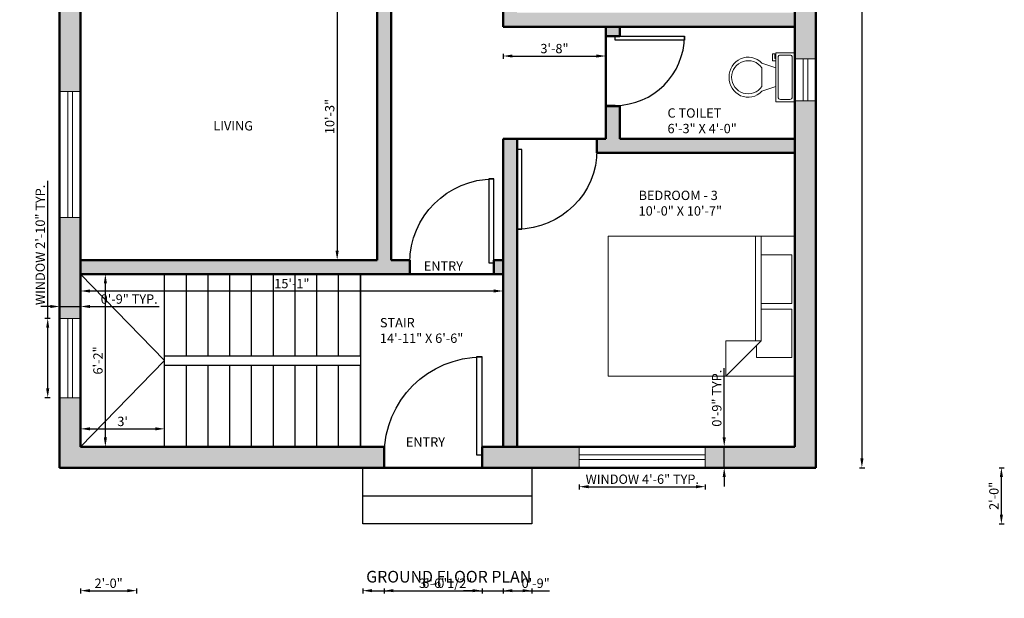
# Model space of a CAD drawing. Units: inches. Extents: x -33 to 405, y -509 to 99.
# Tile 1 of 2: x -16 to 405, y -509 to -262. Entities that reach past the tile are written whole.
import ezdxf

# ---------------------------------------------------------------- set-up
doc = ezdxf.new("R2010")
doc.units = ezdxf.units.IN
for name, color, linetype, lineweight in [('A-ANNO-DIMS', 2, 'Continuous', 18), ('A-ANNO-TEXT', 7, 'Continuous', 25), ('A-AREA-IDEN', 7, 'Continuous', 18), ('A-DOOR', 4, 'Continuous', 25), ('A-FLOR-FIXT', 8, 'Continuous', 18), ('A-FLOR-STRS', 7, 'Continuous', 25), ('A-FURN', 9, 'Continuous', 18), ('A-GLAZ', 6, 'Continuous', 18), ('A-WALL', 7, 'Continuous', 50), ('A-WALL-PATT', 251, 'Continuous', 13)]:
    doc.layers.add(name, color=color, linetype=linetype, lineweight=lineweight)
doc.styles.get("Standard").update_dxf_attribs({"font": 'arial.ttf'})
doc.dimstyles.new('ISO-25', dxfattribs={"dimtxt": 4, "dimasz": 4, "dimexe": 1.25, "dimexo": 0.625, "dimtad": 1, "dimlunit": 3, "dimtxsty": 'Standard', "dimcen": 2.5, "dimadec": 0, "dimazin": 0, "dimtfac": 1, "dimtmove": 0, "dimatfit": 3, "dimfxl": 1, "dimfxlon": 1, "dimarcsym": 0})

# ---------------------------------------------------------------- blocks, each defined once
blk = doc.blocks.new('*U2')
for p, q in [((9.5, -6), (9.5, -2)), ((-8, -8.5), (-8, -8)), ((-7, -8), (-7, -9.5)), ((-4, -8), (-6, -14)), ((4, -8), (6, -14)), ((-10, -8.5), (-8, -8.5)), ((-10, -9.5), (-10, -8.5)), ((-7, -9.5), (-10, -9.5)), ((4, -14), (-4, -14))]:
    blk.add_line(p, q)
blk.add_lwpolyline([(10.5, -8), (10.5, 0), (-10.5, 0), (-10.5, -8)], close=True)
for points in [[(-9.5, -2), (-9.5, -6)], [(8.5, -1), (-8.5, -1)], [(-8.5, -7), (8.5, -7)]]:
    blk.add_lwpolyline(points)
for centre, radius, start, end in [((-8.625, -1.875), 0.8839, 81.8699, 188.1301), ((8.625, -1.875), 0.8839, 351.8699, 98.1301), ((-8.625, -6.125), 0.8839, 171.869898, 278.1301), ((8.625, -6.125), 0.8839, 261.8699, 8.1301), ((-0.4772, -19.9188), 8.0953, 133.01722, 273.38), ((0.0374, -19.8731), 7.127, 124.50543, 269.7), ((-0.0373, -19.8731), 7.127, 270.3, 55.4946), ((0.4773, -19.9188), 8.0953, 266.62, 46.9828)]:
    blk.add_arc(centre, radius, start, end)
blk = doc.blocks.new('*U4')
for p, q in [((0, 0), (0, -100)), ((750, 0), (750, -100))]:
    blk.add_line(p, q)
blk.add_lwpolyline([(0, 0), (0, 750), (43.75, 750), (43.75, 0)], close=True)
blk.add_arc((0, 0), 750, 0, 90)
blk = doc.blocks.new('Bed - Queen')
for p, q in [((0, -80.00003), (0, 0)), ((0, 0), (59.99999, 0)), ((59.99999, 0), (59.99999, -80.00003)), ((7.99999, -1.2), (28.79998, -1.2)), ((7.99999, -14.4), (7.99999, -1.2)), ((28.79998, -1.2), (28.79998, -14.4)), ((31.19999, -1.2), (51.99999, -1.2)), ((31.19999, -14.4), (31.19999, -1.2)), ((51.99999, -1.2), (51.99999, -16.4)), ((0, -14.4), (44.8, -14.4)), ((44.8, -16.8), (0, -16.8)), ((59.99999, -29.6), (44.8, -14.4)), ((44.8, -14.4), (44.8, -29.6)), ((51.99999, -16.4), (46.79936, -16.4)), ((44.8, -29.6), (59.99999, -29.6)), ((59.99999, -80.00003), (0, -80.00003))]:
    blk.add_line(p, q)
blk = doc.blocks.new('*D9')
at = {"layer": 'A-ANNO-DIMS', "color": 0, "lineweight": -2, "transparency": 16777216}
for p, q in [((9.69, -376.8), (9.69, -379.05)), ((13.69, -377.8), (186.69, -377.8)), ((190.69, -376.8), (190.69, -379.05))]:
    blk.add_line(p, q, dxfattribs=at)
at = {"layer": 'A-ANNO-DIMS', "color": 0, "transparency": 16777216}
for points in [[(13.69, -377.13), (13.69, -378.47), (9.69, -377.8)], [(186.69, -377.13), (186.69, -378.47), (190.69, -377.8)]]:
    blk.add_solid(points, dxfattribs=at)
at = {"layer": 'Defpoints', "color": 0, "transparency": 16777216}
for p in [(9.69, -370.55), (190.69, -370.55), (190.69, -377.8)]:
    blk.add_point(p, dxfattribs=at)
at = {"layer": 'A-ANNO-DIMS', "color": 0, "transparency": 16777216, "insert": (100.19, -375.13), "char_height": 4, "attachment_point": 5}
blk.add_mtext('15\'-1"', dxfattribs=at)
blk = doc.blocks.new('*D10')
at = {"layer": 'A-ANNO-DIMS', "color": 0, "lineweight": -2, "transparency": 16777216}
for p, q in [((9.69, -437.87), (9.69, -435.62)), ((13.69, -436.87), (41.69, -436.87)), ((45.69, -437.87), (45.69, -435.62))]:
    blk.add_line(p, q, dxfattribs=at)
at = {"layer": 'A-ANNO-DIMS', "color": 0, "transparency": 16777216}
for points in [[(13.69, -436.2), (13.69, -437.53), (9.69, -436.87)], [(41.69, -436.2), (41.69, -437.53), (45.69, -436.87)]]:
    blk.add_solid(points, dxfattribs=at)
at = {"layer": 'Defpoints', "color": 0, "transparency": 16777216}
for p in [(45.69, -436.87), (9.69, -444.55), (45.69, -444.55)]:
    blk.add_point(p, dxfattribs=at)
at = {"layer": 'A-ANNO-DIMS', "color": 0, "transparency": 16777216, "insert": (27.69, -434.2), "char_height": 4, "attachment_point": 5}
blk.add_mtext("3'", dxfattribs=at)
blk = doc.blocks.new('*D11')
at = {"layer": 'A-ANNO-DIMS', "color": 0, "lineweight": -2, "transparency": 16777216}
for p, q in [((19.29, -370.55), (21.54, -370.55)), ((20.29, -440.55), (20.29, -374.55)), ((19.29, -444.55), (21.54, -444.55))]:
    blk.add_line(p, q, dxfattribs=at)
at = {"layer": 'A-ANNO-DIMS', "color": 0, "transparency": 16777216}
for points in [[(19.63, -374.55), (20.96, -374.55), (20.29, -370.55)], [(19.63, -440.55), (20.96, -440.55), (20.29, -444.55)]]:
    blk.add_solid(points, dxfattribs=at)
at = {"layer": 'Defpoints', "color": 0, "transparency": 16777216}
for p in [(9.69, -370.55), (20.29, -370.55), (9.69, -444.55)]:
    blk.add_point(p, dxfattribs=at)
at = {"layer": 'A-ANNO-DIMS', "color": 0, "transparency": 16777216, "insert": (17.63, -407.55), "char_height": 4, "attachment_point": 5, "rotation": 90}
blk.add_mtext('6\'-2"', dxfattribs=at)
blk = doc.blocks.new('*D13')
at = {"layer": 'A-ANNO-DIMS', "color": 0, "lineweight": -2, "transparency": 16777216}
for p, q in [((120.59, -241.55), (118.34, -241.55)), ((119.59, -245.55), (119.59, -360.55)), ((120.59, -364.55), (118.34, -364.55))]:
    blk.add_line(p, q, dxfattribs=at)
at = {"layer": 'A-ANNO-DIMS', "color": 0, "transparency": 16777216}
for points in [[(118.92, -245.55), (120.26, -245.55), (119.59, -241.55)], [(118.92, -360.55), (120.26, -360.55), (119.59, -364.55)]]:
    blk.add_solid(points, dxfattribs=at)
at = {"layer": 'Defpoints', "color": 0, "transparency": 16777216}
for p in [(125.69, -241.55), (119.59, -364.55), (125.69, -364.55)]:
    blk.add_point(p, dxfattribs=at)
at = {"layer": 'A-ANNO-DIMS', "color": 0, "transparency": 16777216, "insert": (116.92, -303.05), "char_height": 4, "attachment_point": 5, "rotation": 90}
blk.add_mtext('10\'-3"', dxfattribs=at)
blk = doc.blocks.new('*D14')
at = {"layer": 'A-ANNO-DIMS', "color": 0, "lineweight": -2, "transparency": 16777216}
for p, q in [((190.69, -276.11), (190.69, -278.36)), ((194.69, -277.11), (230.69, -277.11)), ((234.69, -276.11), (234.69, -278.36))]:
    blk.add_line(p, q, dxfattribs=at)
at = {"layer": 'A-ANNO-DIMS', "color": 0, "transparency": 16777216}
for points in [[(194.69, -276.45), (194.69, -277.78), (190.69, -277.11)], [(230.69, -276.45), (230.69, -277.78), (234.69, -277.11)]]:
    blk.add_solid(points, dxfattribs=at)
at = {"layer": 'Defpoints', "color": 0, "transparency": 16777216}
for p in [(190.69, -264.55), (234.69, -264.55), (234.69, -277.11)]:
    blk.add_point(p, dxfattribs=at)
at = {"layer": 'A-ANNO-DIMS', "color": 0, "transparency": 16777216, "insert": (212.69, -274.44), "char_height": 4, "attachment_point": 5}
blk.add_mtext('3\'-8"', dxfattribs=at)
blk = doc.blocks.new('*D16')
at = {"layer": 'A-ANNO-DIMS', "color": 0, "lineweight": -2, "transparency": 16777216}
for p, q in [((343.39, 14.45), (345.64, 14.45)), ((344.39, 10.45), (344.39, -449.55)), ((343.39, -453.55), (345.64, -453.55))]:
    blk.add_line(p, q, dxfattribs=at)
at = {"layer": 'A-ANNO-DIMS', "color": 0, "transparency": 16777216}
for points in [[(343.72, 10.45), (345.06, 10.45), (344.39, 14.45)], [(343.72, -449.55), (345.06, -449.55), (344.39, -453.55)]]:
    blk.add_solid(points, dxfattribs=at)
at = {"layer": 'Defpoints', "color": 0, "transparency": 16777216}
for p in [(324.69, 14.45), (324.69, -453.55), (344.39, -453.55)]:
    blk.add_point(p, dxfattribs=at)
at = {"layer": 'A-ANNO-DIMS', "color": 0, "transparency": 16777216, "insert": (341.72, -219.55), "char_height": 4, "attachment_point": 5, "rotation": 90}
blk.add_mtext("39'", dxfattribs=at)
blk = doc.blocks.new('WIN-54IN')
for p, q in [((54, 5.5), (0, 5.5)), ((54, 3.5), (0, 3.5))]:
    blk.add_line(p, q)
blk.add_lwpolyline([(54, 9), (54, 0), (0, 0), (0, 9)], close=True)
blk = doc.blocks.new('WIN-18IN')
for p, q in [((3.5, 18), (3.5, 0)), ((5.5, 18), (5.5, 0))]:
    blk.add_line(p, q)
blk.add_lwpolyline([(9, 18), (9, 0), (0, 0), (0, 18)], close=True)
blk = doc.blocks.new('WIN-34IN')
for p, q in [((3.5, 34), (3.5, 0)), ((5.5, 34), (5.5, 0))]:
    blk.add_line(p, q)
blk.add_lwpolyline([(0, 34), (9, 34), (9, 0), (0, 0)], close=True)
blk = doc.blocks.new('*D20')
at = {"layer": 'A-ANNO-DIMS', "color": 0, "lineweight": -2, "transparency": 16777216}
for p, q in [((223.31, -460.65), (223.31, -462.9)), ((227.31, -461.65), (273.31, -461.65)), ((277.31, -460.65), (277.31, -462.9))]:
    blk.add_line(p, q, dxfattribs=at)
at = {"layer": 'A-ANNO-DIMS', "color": 0, "transparency": 16777216}
for points in [[(227.31, -460.98), (227.31, -462.32), (223.31, -461.65)], [(273.31, -460.98), (273.31, -462.32), (277.31, -461.65)]]:
    blk.add_solid(points, dxfattribs=at)
at = {"layer": 'Defpoints', "color": 0, "transparency": 16777216}
for p in [(223.31, -453.55), (277.31, -453.55), (277.31, -461.65)]:
    blk.add_point(p, dxfattribs=at)
at = {"layer": 'A-ANNO-DIMS', "color": 0, "transparency": 16777216, "insert": (250.31, -458.95), "char_height": 4, "attachment_point": 5}
blk.add_mtext('WINDOW 4\'-6" TYP.', dxfattribs=at)
blk = doc.blocks.new('*D21')
at = {"layer": 'A-ANNO-DIMS', "color": 0, "lineweight": -2, "transparency": 16777216}
for p, q in [((285.41, -440.55), (285.41, -410.92)), ((284.41, -444.55), (286.66, -444.55)), ((285.41, -453.55), (285.41, -444.55)), ((284.41, -453.55), (286.66, -453.55)), ((285.41, -457.55), (285.41, -461.55))]:
    blk.add_line(p, q, dxfattribs=at)
at = {"layer": 'A-ANNO-DIMS', "color": 0, "transparency": 16777216}
for points in [[(284.74, -440.55), (286.08, -440.55), (285.41, -444.55)], [(284.74, -457.55), (286.08, -457.55), (285.41, -453.55)]]:
    blk.add_solid(points, dxfattribs=at)
at = {"layer": 'Defpoints', "color": 0, "transparency": 16777216}
for p in [(277.31, -444.55), (285.41, -444.55), (277.31, -453.55)]:
    blk.add_point(p, dxfattribs=at)
at = {"layer": 'A-ANNO-DIMS', "color": 0, "transparency": 16777216, "insert": (282.74, -423.73), "char_height": 4, "attachment_point": 5, "rotation": 90}
blk.add_mtext('0\'-9" TYP.', dxfattribs=at)
blk = doc.blocks.new('*D24')
at = {"layer": 'A-ANNO-DIMS', "color": 0, "lineweight": -2, "transparency": 16777216}
for p, q in [((-4.41, -389.54), (-4.41, -330.56)), ((-3.41, -389.54), (-5.66, -389.54)), ((-4.41, -419.54), (-4.41, -393.54)), ((-3.41, -423.54), (-5.66, -423.54))]:
    blk.add_line(p, q, dxfattribs=at)
at = {"layer": 'A-ANNO-DIMS', "color": 0, "transparency": 16777216}
for points in [[(-5.08, -393.54), (-3.75, -393.54), (-4.41, -389.54)], [(-5.08, -419.54), (-3.75, -419.54), (-4.41, -423.54)]]:
    blk.add_solid(points, dxfattribs=at)
at = {"layer": 'Defpoints', "color": 0, "transparency": 16777216}
for p in [(-4.41, -389.54), (0.69, -389.54), (0.69, -423.54)]:
    blk.add_point(p, dxfattribs=at)
at = {"layer": 'A-ANNO-DIMS', "color": 0, "transparency": 16777216, "insert": (-7.11, -358.05), "char_height": 4, "attachment_point": 5, "rotation": 90}
blk.add_mtext('WINDOW 2\'-10" TYP.', dxfattribs=at)
blk = doc.blocks.new('*D25')
at = {"layer": 'A-ANNO-DIMS', "color": 0, "lineweight": -2, "transparency": 16777216}
for p, q in [((0.69, -385.44), (0.69, -383.19)), ((9.69, -385.44), (9.69, -383.19)), ((-3.31, -384.44), (-7.31, -384.44)), ((0.69, -384.44), (9.69, -384.44)), ((13.69, -384.44), (43.32, -384.44))]:
    blk.add_line(p, q, dxfattribs=at)
at = {"layer": 'A-ANNO-DIMS', "color": 0, "transparency": 16777216}
for points in [[(-3.31, -383.77), (-3.31, -385.1), (0.69, -384.44)], [(13.69, -383.77), (13.69, -385.1), (9.69, -384.44)]]:
    blk.add_solid(points, dxfattribs=at)
at = {"layer": 'Defpoints', "color": 0, "transparency": 16777216}
for p in [(9.69, -384.44), (0.69, -389.54), (9.69, -389.54)]:
    blk.add_point(p, dxfattribs=at)
at = {"layer": 'A-ANNO-DIMS', "color": 0, "transparency": 16777216, "insert": (30.5, -381.77), "char_height": 4, "attachment_point": 5}
blk.add_mtext('0\'-9" TYP.', dxfattribs=at)
blk = doc.blocks.new('*D34')
at = {"layer": 'A-ANNO-DIMS', "color": 0, "lineweight": -2, "transparency": 16777216}
for p, q in [((130.54, -505.21), (130.54, -507.46)), ((203, -505.21), (203, -507.46)), ((134.54, -506.21), (199, -506.21))]:
    blk.add_line(p, q, dxfattribs=at)
at = {"layer": 'A-ANNO-DIMS', "color": 0, "transparency": 16777216}
for points in [[(134.54, -505.54), (134.54, -506.87), (130.54, -506.21)], [(199, -505.54), (199, -506.87), (203, -506.21)]]:
    blk.add_solid(points, dxfattribs=at)
at = {"layer": 'Defpoints', "color": 0, "transparency": 16777216}
for p in [(130.54, -477.61), (203, -477.61), (203, -506.21)]:
    blk.add_point(p, dxfattribs=at)
at = {"layer": 'A-ANNO-DIMS', "color": 0, "transparency": 16777216, "insert": (166.77, -503.51), "char_height": 4, "attachment_point": 5}
blk.add_mtext('6\'-0 1/2"', dxfattribs=at)
blk = doc.blocks.new('*D35')
at = {"layer": 'A-ANNO-DIMS', "color": 0, "lineweight": -2, "transparency": 16777216}
for p, q in [((403.15, -453.55), (405.4, -453.55)), ((404.15, -473.61), (404.15, -457.55)), ((403.15, -477.61), (405.4, -477.61))]:
    blk.add_line(p, q, dxfattribs=at)
at = {"layer": 'A-ANNO-DIMS', "color": 0, "transparency": 16777216}
for points in [[(403.48, -457.55), (404.82, -457.55), (404.15, -453.55)], [(403.48, -473.61), (404.82, -473.61), (404.15, -477.61)]]:
    blk.add_solid(points, dxfattribs=at)
at = {"layer": 'Defpoints', "color": 0, "transparency": 16777216}
for p in [(203, -453.55), (404.15, -453.55), (203, -477.61)]:
    blk.add_point(p, dxfattribs=at)
at = {"layer": 'A-ANNO-DIMS', "color": 0, "transparency": 16777216, "insert": (401.48, -465.58), "char_height": 4, "attachment_point": 5, "rotation": 90}
blk.add_mtext('2\'-0"', dxfattribs=at)
blk = doc.blocks.new('*D36')
at = {"layer": 'A-ANNO-DIMS', "color": 0, "lineweight": -2, "transparency": 16777216}
for p, q in [((139.69, -505.21), (139.69, -507.46)), ((181.69, -505.21), (181.69, -507.46)), ((143.69, -506.21), (177.69, -506.21))]:
    blk.add_line(p, q, dxfattribs=at)
at = {"layer": 'A-ANNO-DIMS', "color": 0, "transparency": 16777216}
for points in [[(143.69, -505.54), (143.69, -506.87), (139.69, -506.21)], [(177.69, -505.54), (177.69, -506.87), (181.69, -506.21)]]:
    blk.add_solid(points, dxfattribs=at)
at = {"layer": 'Defpoints', "color": 0, "transparency": 16777216}
for p in [(139.69, -453.55), (181.69, -453.55), (181.69, -506.21)]:
    blk.add_point(p, dxfattribs=at)
at = {"layer": 'A-ANNO-DIMS', "color": 0, "transparency": 16777216, "insert": (160.69, -503.54), "char_height": 4, "attachment_point": 5}
blk.add_mtext('3\'-6"', dxfattribs=at)
blk = doc.blocks.new('*D37')
at = {"layer": 'A-ANNO-DIMS', "color": 0, "lineweight": -2, "transparency": 16777216}
for p, q in [((9.69, -505.21), (9.69, -507.46)), ((33.69, -505.21), (33.69, -507.46)), ((13.69, -506.21), (29.69, -506.21))]:
    blk.add_line(p, q, dxfattribs=at)
at = {"layer": 'A-ANNO-DIMS', "color": 0, "transparency": 16777216}
for points in [[(13.69, -505.54), (13.69, -506.87), (9.69, -506.21)], [(29.69, -505.54), (29.69, -506.87), (33.69, -506.21)]]:
    blk.add_solid(points, dxfattribs=at)
at = {"layer": 'Defpoints', "color": 0, "transparency": 16777216}
for p in [(9.69, -89.55), (33.69, -89.55), (33.69, -506.21)]:
    blk.add_point(p, dxfattribs=at)
at = {"layer": 'A-ANNO-DIMS', "color": 0, "transparency": 16777216, "insert": (21.69, -503.54), "char_height": 4, "attachment_point": 5}
blk.add_mtext('2\'-0"', dxfattribs=at)
blk = doc.blocks.new('*D41')
at = {"layer": 'A-ANNO-DIMS', "color": 0, "lineweight": -2, "transparency": 16777216}
for p, q in [((181.69, -505.21), (181.69, -507.46)), ((190.69, -505.21), (190.69, -507.46)), ((177.69, -506.21), (173.69, -506.21)), ((181.69, -506.21), (190.69, -506.21)), ((194.69, -506.21), (210.57, -506.21))]:
    blk.add_line(p, q, dxfattribs=at)
at = {"layer": 'A-ANNO-DIMS', "color": 0, "transparency": 16777216}
for points in [[(177.69, -505.54), (177.69, -506.87), (181.69, -506.21)], [(194.69, -505.54), (194.69, -506.87), (190.69, -506.21)]]:
    blk.add_solid(points, dxfattribs=at)
at = {"layer": 'Defpoints', "color": 0, "transparency": 16777216}
for p in [(181.69, -444.55), (190.69, -444.55), (190.69, -506.21)]:
    blk.add_point(p, dxfattribs=at)
at = {"layer": 'A-ANNO-DIMS', "color": 0, "transparency": 16777216, "insert": (204.63, -503.54), "char_height": 4, "attachment_point": 5}
blk.add_mtext('0\'-9"', dxfattribs=at)

msp = doc.modelspace()

# ---------------------------------------------------------------- hatches: boundary and pattern name
at = {"layer": 'A-WALL-PATT'}
h = msp.add_hatch(color=256, dxfattribs=at)
h.dxf.hatch_style = 1
h.paths.add_polyline_path([(9.686, -48.411), (0.686, -48.411), (0.686, -120.696), (9.686, -120.696)])
h.paths.add_polyline_path([(100.686, 5.451), (94.686, 5.451), (94.686, -50.549), (100.686, -50.549)])
h.paths.add_polyline_path([(142.686, 5.451), (136.686, 5.451), (136.686, -84.549), (142.686, -84.549)])
h.paths.add_polyline_path([(196.686, 5.451), (190.686, 5.451), (190.686, -50.609), (190.777, -50.609, -0.0158204), (192.678, -50.549), (196.686, -50.549)])
h.paths.add_polyline_path([(196.686, -80.609), (192.678, -80.609), (190.686, -80.609), (190.686, -84.549), (100.686, -84.549), (100.686, -80.549), (98.685, -80.549), (94.686, -80.549), (94.686, -90.549), (196.686, -90.549)])
h.paths.add_polyline_path([(324.686, -99.53), (315.686, -99.53), (315.686, -165.584), (324.686, -165.584)])
h.paths.add_polyline_path([(315.686, -126.549), (182.686, -126.549), (182.686, -132.549), (190.686, -132.549), (190.686, -218.549), (196.686, -218.549), (196.686, -132.549), (315.686, -132.549)])
h.paths.add_polyline_path([(142.686, -90.549), (136.686, -90.549), (136.686, -183.549), (94.686, -183.549), (94.686, -187.549), (142.686, -187.549), (142.686, -132.549), (146.686, -132.549), (146.686, -127.759), (146.686, -126.549), (142.686, -126.549)])
h.paths.add_polyline_path([(142.686, -237.549), (94.686, -237.549), (94.686, -241.549), (136.686, -241.549), (136.686, -364.549), (9.686, -364.549), (9.686, -370.549), (136.686, -370.549), (150.686, -370.549), (150.686, -364.549), (142.686, -364.549)])
h.paths.add_polyline_path([(196.686, -312.549), (190.686, -312.549), (190.686, -444.549), (196.686, -444.549)])
h.paths.add_polyline_path([(190.686, -364.549), (186.686, -364.549), (186.686, -365.752), (186.686, -370.549), (190.686, -370.549)])
h.paths.add_polyline_path([(315.686, -312.549), (240.686, -312.549), (240.686, -298.549), (234.686, -298.549), (234.686, -312.549), (230.9, -312.549), (230.9, -317.111, -0.0105112), (230.87, -318.549), (234.686, -318.549), (240.686, -318.549), (315.686, -318.549)])
h.paths.add_polyline_path([(315.686, -258.549), (196.686, -258.549), (196.686, -254.549), (195.477, -254.549), (190.686, -254.549), (190.686, -264.549), (315.686, -264.549)])
h.paths.add_polyline_path([(240.686, -264.549), (234.686, -264.549), (234.686, -268.549), (238.649, -268.549), (240.686, -268.549)])
h.paths.add_polyline_path([(324.686, -296.335), (315.686, -296.335), (315.686, -444.549), (277.309, -444.549), (277.309, -453.549), (324.686, -453.549)])
h.paths.add_polyline_path([(324.686, -219.584), (315.686, -219.584), (315.686, -278.335), (324.686, -278.335)])
h.paths.add_polyline_path([(9.686, -174.696), (0.686, -174.696), (0.686, -292.323), (9.686, -292.323)])
h.paths.add_polyline_path([(9.686, -364.549), (9.686, -346.323), (0.686, -346.323), (0.686, -389.536), (9.686, -389.536), (9.686, -370.549)])
h.paths.add_polyline_path([(139.686, -444.549), (9.686, -444.549), (9.686, -423.536), (0.686, -423.536), (0.686, -453.549), (139.686, -453.549)])
h.paths.add_polyline_path([(223.309, -444.549), (181.686, -444.549), (181.686, -447.962), (181.686, -453.549), (223.309, -453.549)])

# ---------------------------------------------------------------- linework, layer by layer
at = {"layer": 'A-FLOR-STRS'}
for p, q in [((45.686, -407.549), (9.686, -370.549)), ((45.686, -405.549), (45.686, -370.549)), ((55.003, -405.549), (55.003, -370.549)), ((64.321, -405.549), (64.321, -370.549)), ((73.638, -405.549), (73.638, -370.549)), ((82.956, -405.549), (82.956, -370.549)), ((92.273, -405.549), (92.273, -370.549)), ((101.59, -405.549), (101.59, -370.549)), ((110.908, -405.549), (110.908, -370.549)), ((120.225, -405.549), (120.225, -370.549)), ((129.543, -370.549), (129.543, -444.549)), ((129.543, -405.549), (129.543, -370.549)), ((45.686, -407.549), (9.686, -444.549)), ((45.686, -405.549), (129.543, -405.549)), ((45.686, -409.549), (45.686, -405.549)), ((45.686, -444.549), (45.686, -409.549)), ((45.686, -409.549), (129.543, -409.549)), ((55.003, -444.549), (55.003, -409.549)), ((64.321, -444.549), (64.321, -409.549)), ((73.638, -444.549), (73.638, -409.549)), ((82.956, -444.549), (82.956, -409.549)), ((92.273, -444.549), (92.273, -409.549)), ((101.59, -444.549), (101.59, -409.549)), ((110.908, -444.549), (110.908, -409.549)), ((120.225, -444.549), (120.225, -409.549)), ((129.543, -444.549), (129.543, -409.549)), ((130.543, -465.577), (202.999, -465.577))]:
    msp.add_line(p, q, dxfattribs=at)
msp.add_lwpolyline([(130.543, -453.549), (202.999, -453.549), (202.999, -477.605), (130.543, -477.605)], close=True, dxfattribs=at)
at = {"layer": 'A-WALL'}
for p, q in [((0.686, -453.549), (0.686, 14.451)), ((324.686, 14.451), (324.686, -453.549)), ((9.686, -370.549), (9.686, 5.451)), ((315.686, 5.451), (315.686, -444.549)), ((190.686, -264.549), (190.686, -132.549)), ((142.686, -364.549), (142.686, -237.549)), ((136.686, -364.549), (136.686, -241.549)), ((190.686, -264.549), (315.686, -264.549)), ((234.686, -264.549), (234.686, -312.549)), ((240.686, -264.549), (240.686, -268.549)), ((240.686, -268.549), (234.686, -268.549)), ((240.686, -298.549), (234.686, -298.549)), ((240.686, -298.549), (240.686, -312.549)), ((190.686, -444.549), (190.686, -312.549)), ((234.686, -312.549), (190.686, -312.549)), ((196.686, -444.549), (196.686, -312.549)), ((230.856, -312.549), (230.856, -318.549)), ((240.686, -312.549), (315.686, -312.549)), ((234.686, -318.549), (230.856, -318.549)), ((240.686, -318.549), (234.686, -318.549)), ((240.686, -318.549), (315.686, -318.549)), ((136.686, -364.549), (9.686, -364.549)), ((142.686, -364.549), (150.686, -364.549)), ((150.686, -364.549), (150.686, -370.549)), ((186.686, -364.549), (186.686, -370.549)), ((186.686, -364.549), (190.686, -364.549)), ((9.686, -444.549), (9.686, -370.549)), ((136.686, -370.549), (9.686, -370.549)), ((136.686, -370.549), (190.686, -370.549)), ((139.686, -444.549), (9.686, -444.549)), ((139.686, -444.549), (139.686, -453.549)), ((315.686, -444.549), (181.686, -444.549)), ((181.686, -444.549), (181.686, -453.549)), ((324.686, -453.549), (0.686, -453.549))]:
    msp.add_line(p, q, dxfattribs=at)

# ---------------------------------------------------------------- block references
at = {"layer": 'A-DOOR'}
for p, xscale, yscale, zscale, rotation in [((238.649, -268.549), 0.0396324154111602, 0.0396324154111602, 0.0396324154111602, 270), ((196.686, -317.111), -0.0456193696706115, 0.0456193696706115, 0.0456193696706115, 180)]:
    msp.add_blockref('*U4', p, dxfattribs=dict(at, xscale=xscale, yscale=yscale, zscale=zscale, rotation=rotation))
for p, xscale, yscale, zscale in [((186.686, -365.752), -0.0479699444317551, 0.0479699444317551, 0.0479699444317551), ((181.686, -447.962), -0.0558704742903991, 0.0558704742903991, 0.0558704742903991)]:
    msp.add_blockref('*U4', p, dxfattribs=dict(at, xscale=xscale, yscale=yscale, zscale=zscale))
at = {"layer": 'A-FLOR-FIXT', "rotation": 270}
msp.add_blockref('*U2', (315.551, -286.197), dxfattribs=at)
at = {"layer": 'A-FURN', "rotation": 270}
msp.add_blockref('Bed - Queen', (315.64, -354.356), dxfattribs=at)
at = {"layer": 'A-GLAZ'}
for name, p in [('WIN-18IN', (315.686, -296.335)), ('WIN-34IN', (0.686, -423.536)), ('WIN-54IN', (223.309, -453.549))]:
    msp.add_blockref(name, p, dxfattribs=at)
at = {"layer": 'A-GLAZ', "rotation": 90.00000000000018}
msp.add_blockref('WIN-54IN', (9.686, -346.323), dxfattribs=at)

# ---------------------------------------------------------------- texts
at = {"layer": 'A-ANNO-TEXT', "insert": (132.025, -497.708), "char_height": 5, "attachment_point": 1}
msp.add_mtext_dynamic_manual_height_columns('GROUND FLOOR PLAN', width=157.81599, gutter_width=12.5, heights=[0], dxfattribs=at)
at = {"layer": 'A-AREA-IDEN', "char_height": 4, "attachment_point": 1}
for s, width, insert in [('C TOILET\\P6\'-3" X 4\'-0"', 34.59465, (261.111, -299.522)), ('LIVING', 40.18505, (66.542, -305.025)), ('BEDROOM - 3\\P10\'-0" X 10\'-7"', 38.63422, (248.736, -334.825)), ('ENTRY', 21.65777, (156.691, -365.083)), ('STAIR\\P\\pxt4;14\'-11" X 6\'-6"', 43.50422, (137.908, -389.367)), ('ENTRY', 25.23925, (149.016, -440.516))]:
    msp.add_mtext_dynamic_manual_height_columns(s, width=width, gutter_width=12.5, heights=[0], dxfattribs=dict(at, insert=insert))

# ---------------------------------------------------------------- dimensions: what is measured, and where the dimension line sits
at = {"layer": 'A-ANNO-DIMS'}
for base, p1, p2, override, picture, middle in [((344.391, -453.549), (324.686, 14.451), (324.686, -453.549), {"dimclrd": 0, "dimclre": 0, "dimclrt": 0}, '*D16', (341.723, -219.549)), ((119.588, -364.549), (125.691, -241.549), (125.691, -364.549), {"dimclrd": 0, "dimclre": 0, "dimclrt": 0}, '*D13', (116.92, -303.049)), ((20.294, -370.549), (9.686, -444.549), (9.686, -370.549), {"dimclrd": 0, "dimclre": 0, "dimclrt": 0}, '*D11', (17.627, -407.549)), ((404.151, -453.549), (202.999, -477.605), (202.999, -453.549), {"dimdec": 1, "dimlfac": 1, "dimrnd": 0, "dimzin": 1, "dimdsep": 46, "dimlunit": 4, "dimfrac": 2}, '*D35', (401.484, -465.577))]:
    dim = msp.add_linear_dim(base=base, p1=p1, p2=p2, angle=90, dimstyle='ISO-25', override=override, dxfattribs=at)
    dim.commit()
    dim.dimension.update_dxf_attribs({"geometry": picture, "text_midpoint": middle})
for base, p1, p2, override, picture, middle in [((33.686, -506.205), (9.686, -89.549), (33.686, -89.549), {"dimdec": 1, "dimlfac": 1, "dimrnd": 0, "dimzin": 1, "dimdsep": 46, "dimlunit": 4, "dimfrac": 2}, '*D37', (21.686, -503.538)), ((234.686, -277.112), (190.686, -264.549), (234.686, -264.549), {"dimclrd": 0, "dimclre": 0, "dimclrt": 0}, '*D14', (212.686, -274.444)), ((190.686, -377.799), (9.686, -370.549), (190.686, -370.549), {"dimclrd": 0, "dimclre": 0, "dimclrt": 0}, '*D9', (100.186, -375.132)), ((45.686, -436.868), (9.686, -444.549), (45.686, -444.549), {"dimclrd": 0, "dimclre": 0, "dimclrt": 0}, '*D10', (27.686, -434.199)), ((190.686, -506.205), (181.686, -444.549), (190.686, -444.549), {"dimdec": 1, "dimlfac": 1, "dimrnd": 0, "dimzin": 1, "dimdsep": 46, "dimlunit": 4, "dimfrac": 2}, '*D41', (204.627, -503.538)), ((181.686, -506.205), (139.686, -453.549), (181.686, -453.549), {"dimdec": 1, "dimlfac": 1, "dimrnd": 0, "dimzin": 1, "dimdsep": 46, "dimlunit": 4, "dimfrac": 2}, '*D36', (160.686, -503.536)), ((202.999, -506.205), (130.543, -477.605), (202.999, -477.605), {"dimdec": 1, "dimlfac": 1, "dimrnd": 0, "dimzin": 1, "dimdsep": 46, "dimlunit": 4, "dimfrac": 2}, '*D34', (166.771, -503.512))]:
    dim = msp.add_linear_dim(base=base, p1=p1, p2=p2, dimstyle='ISO-25', override=override, dxfattribs=at)
    dim.commit()
    dim.dimension.update_dxf_attribs({"geometry": picture, "text_midpoint": middle})
for base, p1, p2, text, picture, middle in [((-4.414, -389.536), (0.686, -423.536), (0.686, -389.536), 'WINDOW <> TYP.', '*D24', (-7.109, -358.049)), ((285.409, -444.549), (277.309, -453.549), (277.309, -444.549), '<> TYP.', '*D21', (282.742, -423.733))]:
    dim = msp.add_linear_dim(base=base, p1=p1, p2=p2, angle=90, text=text, dimstyle='ISO-25', override={"dimdec": 1, "dimlfac": 1, "dimrnd": 0, "dimzin": 1, "dimdsep": 46, "dimlunit": 4, "dimfrac": 2}, dxfattribs=at)
    dim.commit()
    dim.dimension.update_dxf_attribs({"geometry": picture, "text_midpoint": middle})
for base, p1, p2, text, picture, middle in [((9.686, -384.436), (0.686, -389.536), (9.686, -389.536), '<> TYP.', '*D25', (30.502, -381.769)), ((277.309, -461.649), (223.309, -453.549), (277.309, -453.549), 'WINDOW <> TYP.', '*D20', (250.309, -458.955))]:
    dim = msp.add_linear_dim(base=base, p1=p1, p2=p2, text=text, dimstyle='ISO-25', override={"dimdec": 1, "dimlfac": 1, "dimrnd": 0, "dimzin": 1, "dimdsep": 46, "dimlunit": 4, "dimfrac": 2}, dxfattribs=at)
    dim.commit()
    dim.dimension.update_dxf_attribs({"geometry": picture, "text_midpoint": middle})

doc.saveas('drawing.dxf')
